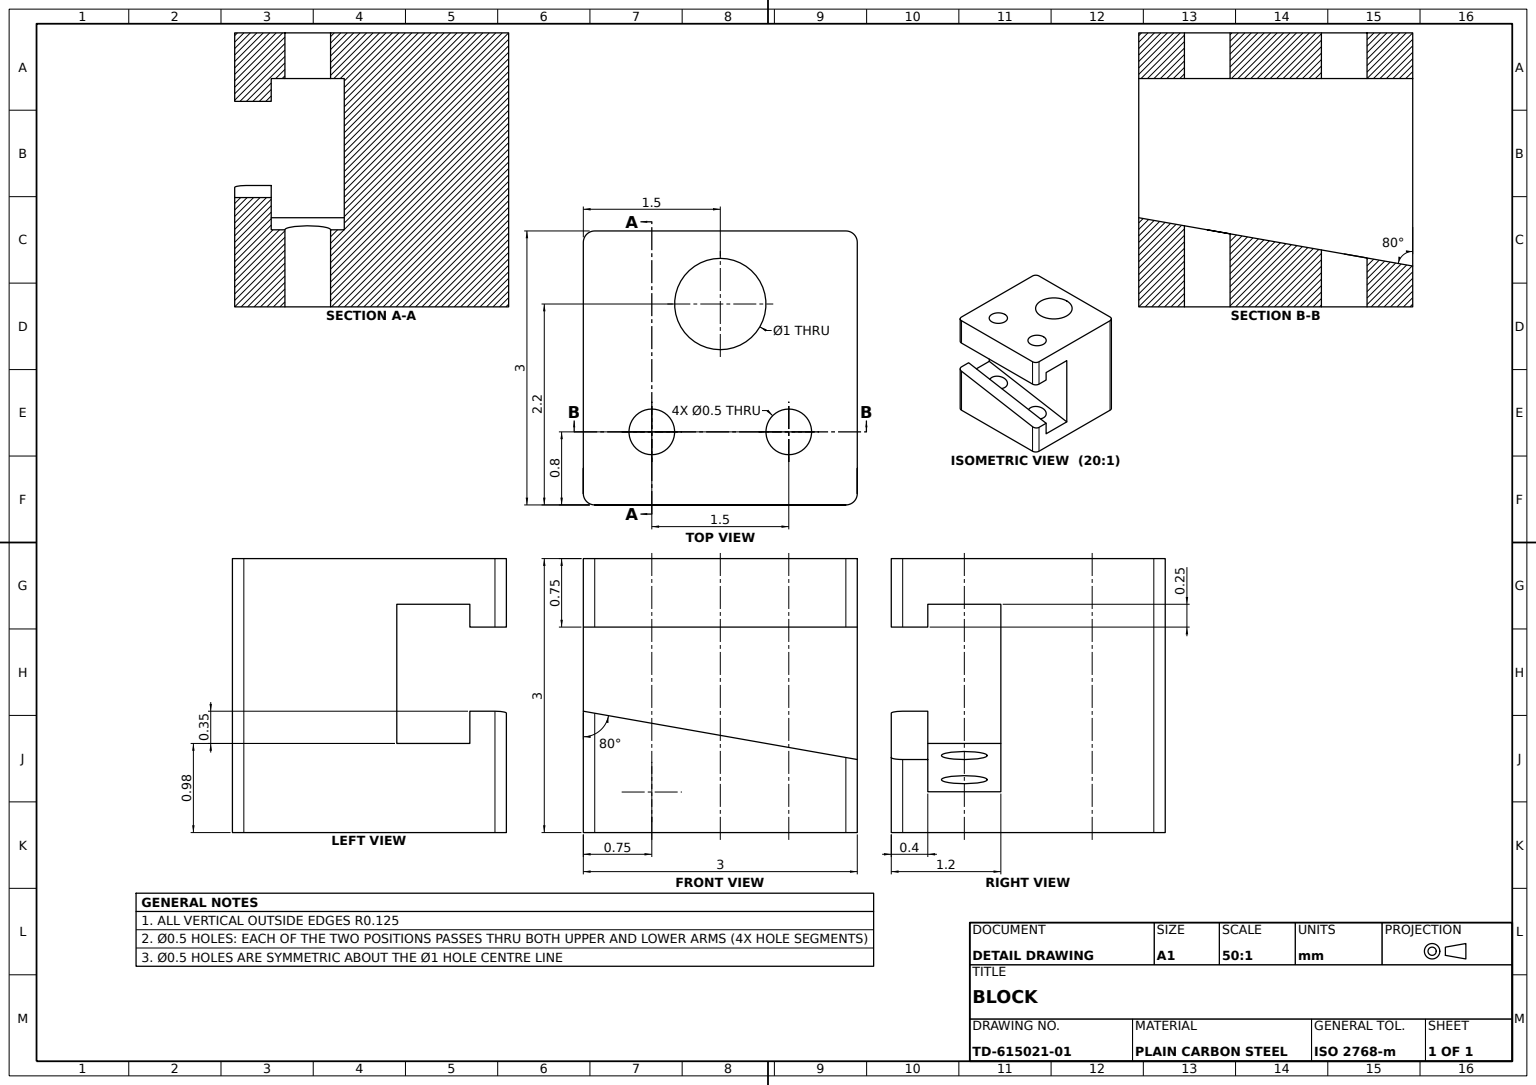
SolidWorks part; units mm, degrees
material "Plain Carbon Steel"
ref_plane "Front Plane" through (0, 0, 0) normal (0, 0, 1) x (1, 0, 0)
ref_plane "Top Plane" through (0, 0, 0) normal (0, 1, 0) x (1, 0, 0)
ref_plane "Right Plane" through (0, 0, 0) normal (1, 0, 0) x (0, 0, -1)
sketch "C-Profile Sketch" plane through (0, 0, 0) normal (0, 0, 1) x (1, 0, 0)
  line L1 (-1.5, 1.5) -> (1.5, 1.5)
  line L2 (-1.5, 1.5) -> (-1.5, -1.5)
  line L3 (-1.5, -1.5) -> (1.5, -1.5)
  line L4 (1.5, 1.5) -> (1.5, -1.5)
  line L5 (-1.5, 1.5) -> (1.5, -1.5) construction
  line L6 (-1.5, -1.5) -> (1.5, 1.5) construction
  point P0 (0, 0)
  dimension "D1" = 3
  dimension "D2" = 3
extrude "C-Body Extrude 3mm" add sketch "C-Profile Sketch" along normal mid plane 3
sketch "Angled Jaw Sketch" plane through (0, 0, 1.5) normal (0, 0, 1) x (1, 0, 0)
  line L0 (1.5, -0.7) -> (-1.5, -0.171)
  line L1 (1.5, -1.5) -> (1.5, 1.5) construction
  line L2 (-1.5, 1.5) -> (-1.5, -1.5) construction
  line L3 (-1.5, 0.75) -> (1.5, 0.75)
  line L4 (1.5, 1.5) -> (-1.5, 1.5) construction
  line L5 (-1.5, 0.75) -> (-1.5, -0.171)
  line L6 (1.5, 0.75) -> (1.5, -0.7)
  line L9 (-1.5, -1.5) -> (1.5, -1.5) construction
  dimension "D1" = 0.75
  dimension "D2" = 0.8
  dimension "D3" = 10
extrude "Angled Jaw Cut 10deg" cut sketch "Angled Jaw Sketch" against normal blind 1.2
sketch "Jaw Notch Sketch" plane through (0, 0, 0.3) normal (0, 0, 1) x (1, 0, 0)
  line L0 (1.5, -0.7) -> (1.5, -1.053)
  line L2 (1.5, -1.5) -> (1.5, -0.7) construction
  line L3 (-1.5, -0.524) -> (1.5, -1.053)
  line L4 (1.5, -0.7) -> (1.5, 1)
  line L5 (1.5, 0.75) -> (1.5, 1.5) construction
  line L6 (1.5, 0.75) -> (-1.5, 0.75) construction
  line L7 (-1.5, -0.524) -> (-1.5, 1)
  line L8 (-1.5, 1.5) -> (-1.5, 0.75) construction
  line L9 (-1.5, 1) -> (1.5, 1)
  line L10 (-1.5, -0.171) -> (-1.5, -1.5) construction
  dimension "D1" = 0.353
  dimension "D2" = 0.25
  dimension "D3" = 80
extrude "Jaw Notch Cut" cut sketch "Jaw Notch Sketch" along normal blind 0.8
fillet "Edge Fillets R0.125" radius 0.125 6 edges at (-1.5, 0, -1.5) (1.5, 0, -1.5) (-1.5, 1.125, 1.5) (-1.5, -0.8355, 1.5) (1.5, 1.125, 1.5) (1.5, -1.1, 1.5)
sketch "Mounting Holes Sketch" plane through (0, 1.5, 0) normal (0, 1, 0) x (1, 0, 0)
  line L0 (-1.5, -1.375) -> (-1.5, 1.375) construction
  line L1 (1.5, -1.375) -> (1.5, 1.375) construction
  line L2 (1.375, -1.5) -> (-1.375, -1.5) construction
  circle A0 centre (0, 0.7) radius 0.5
  circle A1 centre (0.75, -0.7) radius 0.25
  circle A2 centre (-0.75, -0.7) radius 0.25
  dimension "D6" = 1
  dimension "D7" = 0.5
  dimension "D8" = 0.5
  dimension "D1" = 0.75
  dimension "D2" = 0.75
  dimension "D3" = 0.8
  dimension "D4" = 2.2
  dimension "D5" = 1.5
extrude "Mounting Holes 3x" cut sketch "Mounting Holes Sketch" against normal through all
